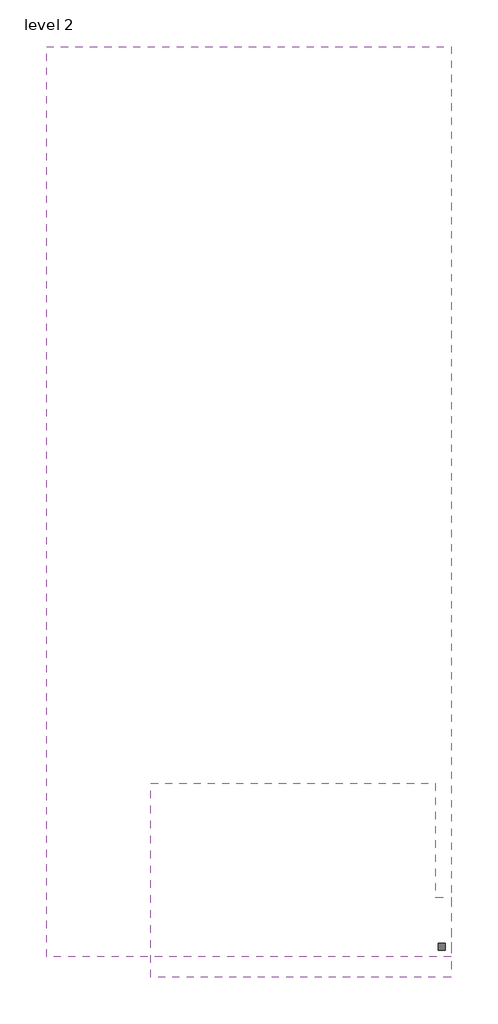
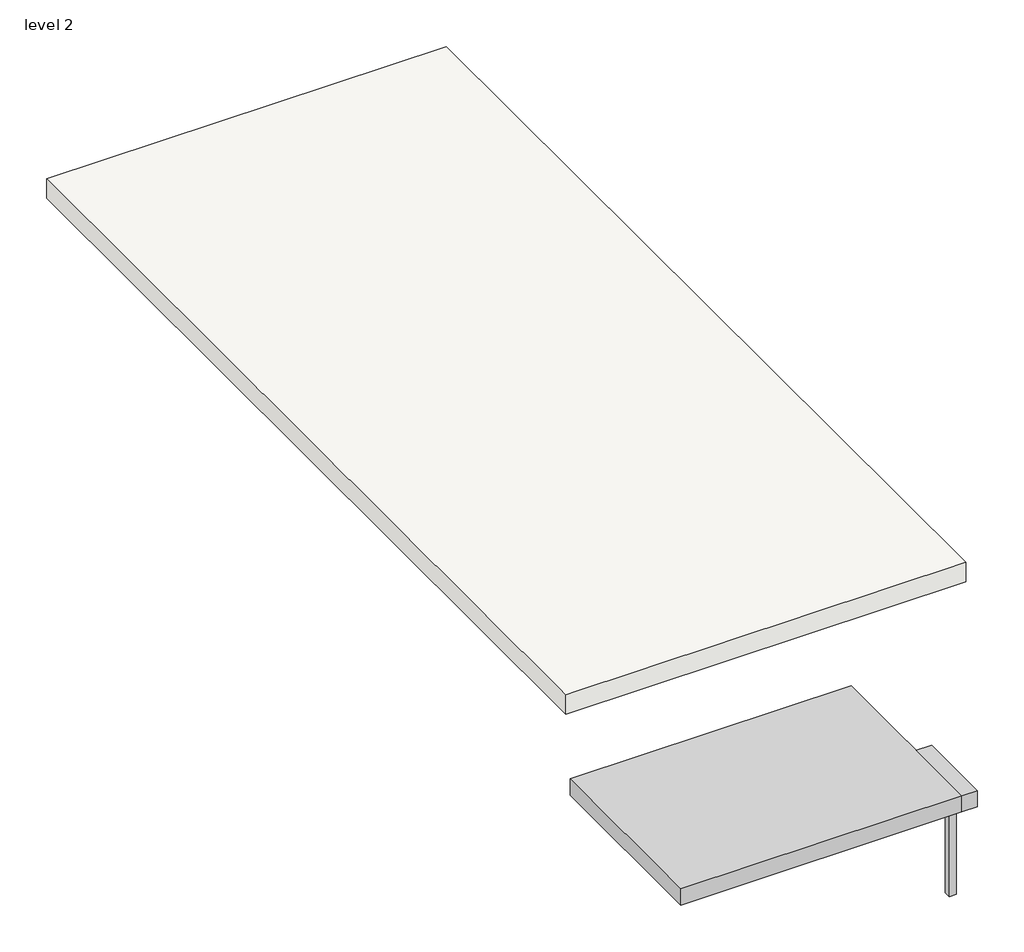
# One storey: 2 proxies, 1 slab.
"""IFC4 building model written with IfcOpenShell, lengths in millimetres."""

from ifc_helpers import new_model, si_unit, frame, origin, place, context, project, spatial, polyline, outline, extrude, transform, mapped, element, save
from components import generic_models_10_generic_models_10_b7097970, generic_models_12_generic_models_12_14ee2a94

model = new_model("IFC4")

# Units and contexts
model_context = context("Model", 3, world=origin())
ifc_project = project(units=[si_unit("LENGTHUNIT", "METRE", prefix="MILLI")], contexts=[model_context])

# Site, building, storey
site = spatial("IfcSite", under=ifc_project)
building = spatial("IfcBuilding", under=site)
storey = spatial("IfcBuildingStorey", under=building, Name="level 2", Elevation=1524.0)

# Proxies
placement = place(None, origin())
generic_models_10_generic_models_10_shape = generic_models_10_generic_models_10_b7097970(model_context)
element("IfcBuildingElementProxy", 1, Name="Generic Models 10 : Generic Models 10", ObjectType="Generic Models 10 : Generic Models 10", at=placement, inside=storey, context=model_context, shape_type="MappedRepresentation", body=[
    mapped(generic_models_10_generic_models_10_shape, transform((0.0, 0.0, 0.0), x_axis=(1.0, 0.0, 0.0), y_axis=(0.0, 1.0, 0.0), z_axis=(0.0, 0.0, 1.0))),
])
generic_models_12_generic_models_12_shape = generic_models_12_generic_models_12_14ee2a94(model_context)
element("IfcBuildingElementProxy", 2, Name="Generic Models 12 : Generic Models 12", ObjectType="Generic Models 12 : Generic Models 12", at=placement, inside=storey, context=model_context, shape_type="MappedRepresentation", body=[
    mapped(generic_models_12_generic_models_12_shape, transform((0.0, 0.0, 0.0), x_axis=(1.0, 0.0, 0.0), y_axis=(0.0, 1.0, 0.0), z_axis=(0.0, 0.0, 1.0))),
])

# Slab
element("IfcSlab", 3, ObjectType="slab 6\"", at=placement, inside=storey, context=model_context, shape_type="SweptSolid", body=[
    extrude(outline(polyline([(-10521.0371373, 9903.938593), (-10521.0371373, -3380.261407), (-16426.5371373, -3380.261407), (-16426.5371373, 9903.938593), (-10521.0371373, 9903.938593)])), frame((0.0, 0.0, 6426.2), z_axis=(0.0, 0.0, 1.0), x_axis=(1.0, 0.0, 0.0)), (0.0, 0.0, 1.0), 304.8),
])

save(model, "model.ifc")

# Revit data of these elements
# Type "slab 6\""
#   Assembly Code = "B1010"
#   Function = 0
#   Layers, outside or top first: 1' - 0" no material (function 1)
# Element 1 (IfcBuildingElementProxy, "Generic Models 10 : Generic Models 10")
#   Phase Created = New Construction
#   Materials on its faces: "Gypsum Wall Board"
# Element 2 (IfcBuildingElementProxy, "Generic Models 12 : Generic Models 12")
#   Phase Created = New Construction
#   Materials on its faces: "Steel, Carbon"
# Element 3 (IfcSlab, "slab 6\"")
#   Height Offset From Level = 17' - 1"
#   Phase Created = New Construction
#   Materials on its faces: "1. WALL PAINT", "Default Floor"
# Materials
#   "Gypsum Wall Board": class "Generic", colour RGB 127 127 127, transparency 0, Description = "Gypsum Wall Board", Cost = 0
#   "Steel, Carbon": class "Metal", colour RGB 0 0 0, transparency 0, Description = "Carbon steel", Cost = 0
#   "1. WALL PAINT": class "Generic", colour RGB 120 120 120, transparency 0, Cost = 0
#   "Default Floor": colour RGB 128 128 128, transparency 0, Cost = 0
